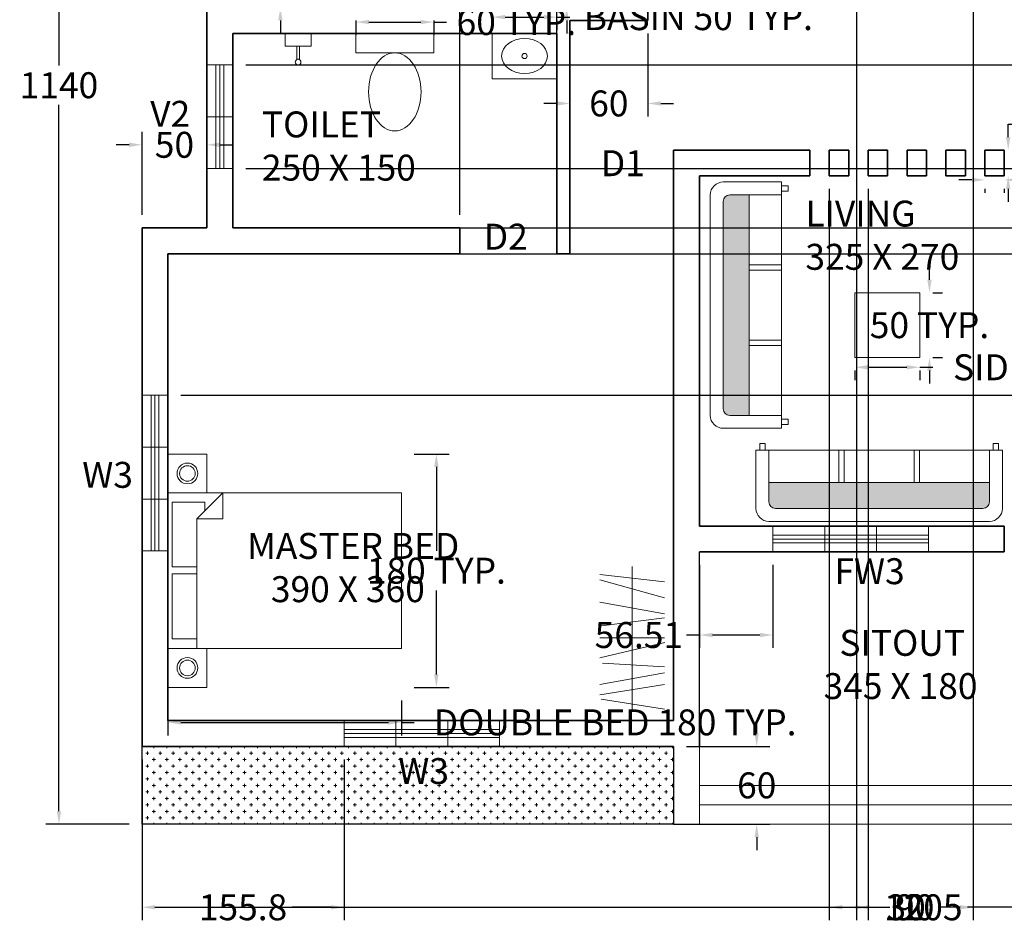
# Model space of a CAD drawing. Units: centimetres. Extents: x 543 to 2148, y 348 to 1642.
# Tile 1 of 4: x 543 to 1302, y 348 to 1046. Entities that reach past the tile are written whole.
import ezdxf

# ---------------------------------------------------------------- set-up
doc = ezdxf.new("R2010")
doc.units = ezdxf.units.CM
doc.header["$MEASUREMENT"] = 0
for name, color, linetype, lineweight in [('A-ANNO-DIMS', 2, 'Continuous', 18), ('A-ANNO-TEXT', 7, 'Continuous', 18), ('A-AREA-IDEN', 7, 'Continuous', 25), ('A-FLOR', 7, 'Continuous', 25), ('A-FLOR-CASE', 8, 'Continuous', 20), ('A-FLOR-FIXT', 8, 'Continuous', 18), ('A-FLOR-PATT', 252, 'Continuous', 13), ('A-FLOR-STRS', 7, 'Continuous', 20), ('A-FURN', 8, 'Continuous', 18), ('A-FURN-PATT', 252, 'Continuous', 13), ('A-GLAZ', 4, 'Continuous', 18), ('A-WALL', 7, 'Continuous', 35)]:
    doc.layers.add(name, color=color, linetype=linetype, lineweight=lineweight)
doc.styles.get("Standard").update_dxf_attribs({"font": 'arial.ttf'})
doc.dimstyles.get("Standard").update_dxf_attribs({"dimtxt": 20, "dimasz": 10, "dimexe": 10, "dimexo": 10, "dimgap": 5, "dimtad": 0, "dimtih": 1, "dimtoh": 1, "dimdec": 0, "dimzin": 0, "dimdsep": 46, "dimtxsty": 'Standard', "dimcen": 5, "dimadec": 0, "dimazin": 0, "dimtfac": 1, "dimtdec": 0, "dimtofl": 0, "dimtmove": 0, "dimatfit": 3, "dimfxl": 1, "dimtolj": 1, "dimtzin": 0, "dimarcsym": 0})

# ---------------------------------------------------------------- blocks, each defined once
blk = doc.blocks.new('BED-DOUBLE')
for p, q in [((42.36, 150), (22.36, 130)), ((42.36, 130), (42.36, 150)), ((22.36, 130), (22.36, 30)), ((22.36, 130), (42.36, 130)), ((3.32, 102.87), (3.32, 92.87)), ((3.32, 92.87), (22.36, 92.87)), ((3.32, 77.49), (3.32, 87.49)), ((3.32, 87.49), (22.36, 87.49))]:
    blk.add_line(p, q)
for points in [[(0, 150), (30, 150), (30, 180), (0, 180)], [(180, 150), (180, 30), (0, 30), (0, 150)], [(0, 0), (30, 0), (30, 30), (0, 30)]]:
    blk.add_lwpolyline(points, close=True)
for points in [[(3.32, 102.87), (3.32, 142.87), (28.32, 142.87), (28.32, 135.96)], [(22.36, 37.49), (3.32, 37.49), (3.32, 77.49)]]:
    blk.add_lwpolyline(points)
for centre, radius in [((15, 165), 8), ((15, 165), 6), ((15, 15), 8), ((15, 15), 6)]:
    blk.add_circle(centre, radius)
blk = doc.blocks.new('SOFA-3SEAT')
for p, q in [((10, 190), (55, 190)), ((55, 190), (55, 125.56)), ((55, 190), (55, 187)), ((55, 187), (60, 187)), ((60, 183), (55, 183)), ((60, 187), (60, 183)), ((0, 125.56), (0, 180)), ((10, 125.56), (10, 175)), ((15, 180), (55, 180)), ((30, 125.56), (30, 180)), ((0, 10), (0, 125.56)), ((10, 15), (10, 125.56)), ((55, 126), (30, 126)), ((30, 10), (30, 125.56)), ((55, 122), (30, 122)), ((55, 125.56), (55, 0)), ((55, 68), (30, 68)), ((55, 64), (30, 64)), ((55, 10), (15, 10)), ((55, 0), (10, 0)), ((60, 7), (55, 7)), ((55, 0), (55, 3)), ((55, 3), (60, 3)), ((60, 3), (60, 7))]:
    blk.add_line(p, q)
for centre, radius, start, end in [((10, 180), 10, 90, 180), ((15, 175), 5, 90, 180), ((10, 10), 10, 180, 270), ((15, 15), 5, 180, 270)]:
    blk.add_arc(centre, radius, start, end)
blk = doc.blocks.new('WARDROBE-RAIL')
for p, q in [((0, 0.31), (7.78, 49.18)), ((11.01, 50.31), (19.09, 0.31)), ((19.09, 50.31), (28.16, 0.3)), ((32.55, 0.31), (35.53, 48.25)), ((39.55, 50.31), (51.34, 0)), ((55, 0.31), (55, 50.31)), ((64.34, 49.01), (70.51, 0.27)), ((73.48, 0.31), (82.64, 50.31)), ((99.87, 50.31), (85.87, 0.31)), ((98.25, 0.31), (103.96, 50.31)), ((0, 25.31), (110, 25.31))]:
    blk.add_line(p, q)
blk = doc.blocks.new('WIN-1200')
for p, q in [((40, 20), (40, 0)), ((80, 20), (80, 0)), ((0, 13), (120, 13)), ((0, 10), (120, 10)), ((0, 7), (120, 7))]:
    blk.add_line(p, q)
blk.add_lwpolyline([(0, 20), (120, 20), (120, 0), (0, 0)], close=True)
blk = doc.blocks.new('VENT-800')
for p, q in [((7, 80), (7, 0)), ((10, 80), (10, 0)), ((13, 80), (13, 0)), ((20, 40), (0, 40)), ((20, 0), (0, 0))]:
    blk.add_line(p, q)
blk.add_lwpolyline([(0, 0), (0, 80), (20, 80), (20, 0)])
blk = doc.blocks.new('WC')
blk.add_lwpolyline([(60, 0), (0, 0), (0, 15), (60, 15)], close=True)
blk.add_ellipse((30, 45.11), major_axis=(0, 30.11), ratio=0.671585)
blk = doc.blocks.new('WASHBASIN')
blk.add_lwpolyline([(50, 0), (0, 0), (0, 35), (50, 35)], close=True)
blk.add_circle((25, 17.5), 2)
blk.add_ellipse((25, 17.5), major_axis=(17.65, 0), ratio=0.767259)
blk = doc.blocks.new('WALL-TAP')
for p, q in [((9, 10), (9, 20)), ((9, 20), (11, 20)), ((11, 10), (11, 20))]:
    blk.add_line(p, q)
blk.add_lwpolyline([(0, 0), (20, 0), (20, 10), (0, 10)], close=True)
blk.add_circle((10, 22.21), 2.21)
blk = doc.blocks.new('TABLE-SIDE')
blk.add_lwpolyline([(0, 50), (50, 50), (50, 0), (0, 0)], close=True)
blk = doc.blocks.new('SCREEN-POST-150X200')
for p, q in [((0, 0), (0, 20)), ((15, 20), (0, 20)), ((15, 0), (15, 20)), ((15, 0), (0, 0))]:
    blk.add_line(p, q)
blk = doc.blocks.new('*D17')
at = {"layer": 'A-ANNO-DIMS', "color": 0, "lineweight": -2, "transparency": 16777216}
for p, q in [((1305.14, 955.09), (1305.14, 965.09)), ((1305.14, 965.09), (1315.14, 965.09)), ((1312.14, 945.09), (1315.14, 945.09)), ((1312.14, 925.09), (1315.14, 925.09)), ((1305.14, 915.09), (1305.14, 905.09))]:
    blk.add_line(p, q, dxfattribs=at)
at = {"layer": 'A-ANNO-DIMS', "color": 0, "transparency": 16777216}
for points in [[(1303.47, 955.09), (1306.81, 955.09), (1305.14, 945.09)], [(1303.47, 915.09), (1306.81, 915.09), (1305.14, 925.09)]]:
    blk.add_solid(points, dxfattribs=at)
at = {"layer": 'Defpoints', "color": 0, "transparency": 16777216}
for p in [(1302.14, 945.09), (1305.14, 945.09), (1302.14, 925.09)]:
    blk.add_point(p, dxfattribs=at)
at = {"layer": 'A-ANNO-DIMS', "color": 0, "transparency": 16777216, "insert": (1472.79, 965.09), "char_height": 20, "attachment_point": 5}
blk.add_mtext('\\A1;SCREEN POST 20 TYP.', dxfattribs=at)
blk = doc.blocks.new('*D18')
at = {"layer": 'A-ANNO-DIMS', "color": 0, "lineweight": -2, "transparency": 16777216}
for p, q in [((1277.14, 922.09), (1267.14, 922.09)), ((1312.14, 922.09), (1322.14, 922.09)), ((1287.14, 915.09), (1287.14, 912.09)), ((1302.14, 915.09), (1302.14, 912.09))]:
    blk.add_line(p, q, dxfattribs=at)
at = {"layer": 'A-ANNO-DIMS', "color": 0, "transparency": 16777216}
for points in [[(1277.14, 923.76), (1277.14, 920.43), (1287.14, 922.09)], [(1312.14, 923.76), (1312.14, 920.43), (1302.14, 922.09)]]:
    blk.add_solid(points, dxfattribs=at)
at = {"layer": 'Defpoints', "color": 0, "transparency": 16777216}
for p in [(1287.14, 925.09), (1302.14, 925.09), (1302.14, 922.09)]:
    blk.add_point(p, dxfattribs=at)
at = {"layer": 'A-ANNO-DIMS', "color": 0, "transparency": 16777216, "insert": (1374.88, 922.09), "char_height": 20, "attachment_point": 5}
blk.add_mtext('\\A1;15 TYP.', dxfattribs=at)
blk = doc.blocks.new('*D21')
at = {"layer": 'A-ANNO-DIMS', "color": 0, "lineweight": -2, "transparency": 16777216}
for p, q in [((657.14, 520.66), (657.14, 493.66)), ((837.14, 520.66), (837.14, 493.66)), ((667.14, 503.66), (827.14, 503.66)), ((837.14, 503.66), (847.14, 503.66))]:
    blk.add_line(p, q, dxfattribs=at)
at = {"layer": 'A-ANNO-DIMS', "color": 0, "transparency": 16777216}
for points in [[(667.14, 505.32), (667.14, 501.99), (657.14, 503.66)], [(827.14, 505.32), (827.14, 501.99), (837.14, 503.66)]]:
    blk.add_solid(points, dxfattribs=at)
at = {"layer": 'Defpoints', "color": 0, "transparency": 16777216}
for p in [(657.14, 530.66), (837.14, 530.66), (837.14, 503.66)]:
    blk.add_point(p, dxfattribs=at)
at = {"layer": 'A-ANNO-DIMS', "color": 0, "transparency": 16777216, "insert": (1002.02, 503.66), "char_height": 20, "attachment_point": 5}
blk.add_mtext('\\A1;DOUBLE BED 180 TYP.', dxfattribs=at)
blk = doc.blocks.new('*D22')
at = {"layer": 'A-ANNO-DIMS', "color": 0, "lineweight": -2, "transparency": 16777216}
for p, q in [((847.14, 710.66), (874.14, 710.66)), ((864.14, 700.66), (864.14, 635.87)), ((864.14, 540.66), (864.14, 605.45)), ((847.14, 530.66), (874.14, 530.66))]:
    blk.add_line(p, q, dxfattribs=at)
at = {"layer": 'A-ANNO-DIMS', "color": 0, "transparency": 16777216}
for points in [[(862.47, 700.66), (865.81, 700.66), (864.14, 710.66)], [(862.47, 540.66), (865.81, 540.66), (864.14, 530.66)]]:
    blk.add_solid(points, dxfattribs=at)
at = {"layer": 'Defpoints', "color": 0, "transparency": 16777216}
for p in [(837.14, 710.66), (864.14, 710.66), (837.14, 530.66)]:
    blk.add_point(p, dxfattribs=at)
at = {"layer": 'A-ANNO-DIMS', "color": 0, "transparency": 16777216, "insert": (864.14, 620.66), "char_height": 20, "attachment_point": 5}
blk.add_mtext('\\A1;180 TYP.', dxfattribs=at)
blk = doc.blocks.new('*D30')
at = {"layer": 'A-ANNO-DIMS', "color": 0, "lineweight": -2, "transparency": 16777216}
for p, q in [((802.08, 1045.09), (802.08, 1033.81)), ((812.08, 1043.81), (852.08, 1043.81)), ((862.08, 1045.09), (862.08, 1033.81)), ((862.08, 1043.81), (872.08, 1043.81))]:
    blk.add_line(p, q, dxfattribs=at)
at = {"layer": 'A-ANNO-DIMS', "color": 0, "transparency": 16777216}
for points in [[(812.08, 1045.47), (812.08, 1042.14), (802.08, 1043.81)], [(852.08, 1045.47), (852.08, 1042.14), (862.08, 1043.81)]]:
    blk.add_solid(points, dxfattribs=at)
at = {"layer": 'Defpoints', "color": 0, "transparency": 16777216}
for p in [(802.08, 1055.09), (862.08, 1055.09), (862.08, 1043.81)]:
    blk.add_point(p, dxfattribs=at)
at = {"layer": 'A-ANNO-DIMS', "color": 0, "transparency": 16777216, "insert": (925.81, 1043.81), "char_height": 20, "attachment_point": 5}
blk.add_mtext('\\A1;60 TYP.', dxfattribs=at)
blk = doc.blocks.new('*D31')
at = {"layer": 'A-ANNO-DIMS', "color": 0, "lineweight": -2, "transparency": 16777216}
for p, q in [((907.14, 1045.09), (907.14, 1037.59)), ((917.14, 1047.59), (947.14, 1047.59)), ((957.14, 1047.59), (967.14, 1047.59)), ((957.14, 1045.09), (957.14, 1037.59))]:
    blk.add_line(p, q, dxfattribs=at)
at = {"layer": 'A-ANNO-DIMS', "color": 0, "transparency": 16777216}
for points in [[(917.14, 1049.26), (917.14, 1045.93), (907.14, 1047.59)], [(947.14, 1049.26), (947.14, 1045.93), (957.14, 1047.59)]]:
    blk.add_solid(points, dxfattribs=at)
at = {"layer": 'Defpoints', "color": 0, "transparency": 16777216}
for p in [(907.14, 1055.09), (957.14, 1055.09), (957.14, 1047.59)]:
    blk.add_point(p, dxfattribs=at)
at = {"layer": 'A-ANNO-DIMS', "color": 0, "transparency": 16777216, "insert": (1066.18, 1047.59), "char_height": 20, "attachment_point": 5}
blk.add_mtext('\\A1;BASIN 50 TYP.', dxfattribs=at)
blk = doc.blocks.new('*D32')
at = {"layer": 'A-ANNO-DIMS', "color": 0, "lineweight": -2, "transparency": 16777216}
for p, q in [((964.64, 1100.09), (964.64, 1110.09)), ((967.14, 1090.09), (974.64, 1090.09)), ((967.14, 1055.09), (974.64, 1055.09)), ((964.64, 1045.09), (964.64, 1035.09))]:
    blk.add_line(p, q, dxfattribs=at)
at = {"layer": 'A-ANNO-DIMS', "color": 0, "transparency": 16777216}
for points in [[(962.97, 1100.09), (966.31, 1100.09), (964.64, 1090.09)], [(962.97, 1045.09), (966.31, 1045.09), (964.64, 1055.09)]]:
    blk.add_solid(points, dxfattribs=at)
at = {"layer": 'Defpoints', "color": 0, "transparency": 16777216}
for p in [(957.14, 1090.09), (964.64, 1090.09), (957.14, 1055.09)]:
    blk.add_point(p, dxfattribs=at)
at = {"layer": 'A-ANNO-DIMS', "color": 0, "transparency": 16777216, "insert": (964.64, 1072.59), "char_height": 20, "attachment_point": 5}
blk.add_mtext('\\A1;35 TYP.', dxfattribs=at)
blk = doc.blocks.new('*D33')
at = {"layer": 'A-ANNO-DIMS', "color": 0, "lineweight": -2, "transparency": 16777216}
for p, q in [((743.83, 1089.51), (743.83, 1099.51)), ((743.83, 1099.51), (753.83, 1099.51)), ((737.5, 1079.51), (733.83, 1079.51)), ((737.5, 1055.09), (733.83, 1055.09)), ((743.83, 1045.09), (743.83, 1035.09))]:
    blk.add_line(p, q, dxfattribs=at)
at = {"layer": 'A-ANNO-DIMS', "color": 0, "transparency": 16777216}
for points in [[(742.17, 1089.51), (745.5, 1089.51), (743.83, 1079.51)], [(742.17, 1045.09), (745.5, 1045.09), (743.83, 1055.09)]]:
    blk.add_solid(points, dxfattribs=at)
at = {"layer": 'Defpoints', "color": 0, "transparency": 16777216}
for p in [(743.83, 1079.51), (747.5, 1079.51), (747.5, 1055.09)]:
    blk.add_point(p, dxfattribs=at)
at = {"layer": 'A-ANNO-DIMS', "color": 0, "transparency": 16777216, "insert": (838.81, 1099.51), "char_height": 20, "attachment_point": 5}
blk.add_mtext('\\A1;TAP 24 TYP.', dxfattribs=at)
blk = doc.blocks.new('*D35')
at = {"layer": 'A-ANNO-DIMS', "color": 0, "lineweight": -2, "transparency": 16777216}
for p, q in [((1186.93, 775.04), (1186.93, 767.54)), ((1196.93, 777.54), (1226.93, 777.54)), ((1236.93, 777.54), (1246.93, 777.54)), ((1236.93, 775.04), (1236.93, 767.54))]:
    blk.add_line(p, q, dxfattribs=at)
at = {"layer": 'A-ANNO-DIMS', "color": 0, "transparency": 16777216}
for points in [[(1196.93, 779.21), (1196.93, 775.87), (1186.93, 777.54)], [(1226.93, 779.21), (1226.93, 775.87), (1236.93, 777.54)]]:
    blk.add_solid(points, dxfattribs=at)
at = {"layer": 'Defpoints', "color": 0, "transparency": 16777216}
for p in [(1186.93, 785.04), (1236.93, 785.04), (1236.93, 777.54)]:
    blk.add_point(p, dxfattribs=at)
at = {"layer": 'A-ANNO-DIMS', "color": 0, "transparency": 16777216, "insert": (1385.19, 777.54), "char_height": 20, "attachment_point": 5}
blk.add_mtext('\\A1;SIDE TABLE 50 TYP.', dxfattribs=at)
blk = doc.blocks.new('*D36')
at = {"layer": 'A-ANNO-DIMS', "color": 0, "lineweight": -2, "transparency": 16777216}
for p, q in [((1244.43, 845.04), (1244.43, 855.04)), ((1246.93, 835.04), (1254.43, 835.04)), ((1246.93, 785.04), (1254.43, 785.04)), ((1244.43, 775.04), (1244.43, 765.04))]:
    blk.add_line(p, q, dxfattribs=at)
at = {"layer": 'A-ANNO-DIMS', "color": 0, "transparency": 16777216}
for points in [[(1242.77, 845.04), (1246.1, 845.04), (1244.43, 835.04)], [(1242.77, 775.04), (1246.1, 775.04), (1244.43, 785.04)]]:
    blk.add_solid(points, dxfattribs=at)
at = {"layer": 'Defpoints', "color": 0, "transparency": 16777216}
for p in [(1236.93, 835.04), (1244.43, 835.04), (1236.93, 785.04)]:
    blk.add_point(p, dxfattribs=at)
at = {"layer": 'A-ANNO-DIMS', "color": 0, "transparency": 16777216, "insert": (1244.43, 810.04), "char_height": 20, "attachment_point": 5}
blk.add_mtext('\\A1;50 TYP.', dxfattribs=at)
blk = doc.blocks.new('*D37')
at = {"layer": 'A-ANNO-DIMS', "color": 0, "lineweight": -2, "transparency": 16777216}
for p, q in [((637.14, 895.09), (637.14, 959.14)), ((687.14, 895.09), (687.14, 959.14)), ((627.14, 949.14), (617.14, 949.14)), ((697.14, 949.14), (707.14, 949.14))]:
    blk.add_line(p, q, dxfattribs=at)
at = {"layer": 'A-ANNO-DIMS', "color": 0, "transparency": 16777216}
for points in [[(627.14, 950.81), (627.14, 947.48), (637.14, 949.14)], [(697.14, 950.81), (697.14, 947.48), (687.14, 949.14)]]:
    blk.add_solid(points, dxfattribs=at)
at = {"layer": 'Defpoints', "color": 0, "transparency": 16777216}
for p in [(687.14, 949.14), (637.14, 885.09), (687.14, 885.09)]:
    blk.add_point(p, dxfattribs=at)
at = {"layer": 'A-ANNO-DIMS', "color": 0, "transparency": 16777216, "insert": (662.14, 949.14), "char_height": 20, "attachment_point": 5}
blk.add_mtext('\\A1;50', dxfattribs=at)
blk = doc.blocks.new('*D44')
at = {"layer": 'A-ANNO-DIMS', "color": 0, "lineweight": -2, "transparency": 16777216}
for p, q in [((882.14, 895.09), (882.14, 1639.14)), ((957.14, 895.09), (957.14, 1639.14)), ((892.14, 1629.14), (900.32, 1629.14)), ((947.14, 1629.14), (938.96, 1629.14))]:
    blk.add_line(p, q, dxfattribs=at)
at = {"layer": 'A-ANNO-DIMS', "color": 0, "transparency": 16777216}
for points in [[(892.14, 1630.81), (892.14, 1627.48), (882.14, 1629.14)], [(947.14, 1630.81), (947.14, 1627.48), (957.14, 1629.14)]]:
    blk.add_solid(points, dxfattribs=at)
at = {"layer": 'Defpoints', "color": 0, "transparency": 16777216}
for p in [(957.14, 1629.14), (882.14, 885.09), (957.14, 885.09)]:
    blk.add_point(p, dxfattribs=at)
at = {"layer": 'A-ANNO-DIMS', "color": 0, "transparency": 16777216, "insert": (919.64, 1629.14), "char_height": 20, "attachment_point": 5}
blk.add_mtext('\\A1;75', dxfattribs=at)
blk = doc.blocks.new('*D46')
at = {"layer": 'A-ANNO-DIMS', "color": 0, "lineweight": -2, "transparency": 16777216}
for p, q in [((1111.19, 495.09), (1111.19, 505.09)), ((1057.14, 485.09), (1121.19, 485.09)), ((1057.14, 425.09), (1121.19, 425.09)), ((1111.19, 415.09), (1111.19, 405.09))]:
    blk.add_line(p, q, dxfattribs=at)
at = {"layer": 'A-ANNO-DIMS', "color": 0, "transparency": 16777216}
for points in [[(1109.52, 495.09), (1112.86, 495.09), (1111.19, 485.09)], [(1109.52, 415.09), (1112.86, 415.09), (1111.19, 425.09)]]:
    blk.add_solid(points, dxfattribs=at)
at = {"layer": 'Defpoints', "color": 0, "transparency": 16777216}
for p in [(1047.14, 485.09), (1047.14, 425.09), (1111.19, 425.09)]:
    blk.add_point(p, dxfattribs=at)
at = {"layer": 'A-ANNO-DIMS', "color": 0, "transparency": 16777216, "insert": (1111.19, 455.09), "char_height": 20, "attachment_point": 5}
blk.add_mtext('\\A1;60', dxfattribs=at)
blk = doc.blocks.new('*D55')
at = {"layer": 'A-ANNO-DIMS', "color": 0, "lineweight": -2, "transparency": 16777216}
for p, q in [((1067.14, 625.09), (1067.14, 561.04)), ((1123.65, 625.09), (1123.65, 561.04)), ((1067.14, 571.04), (1057.14, 571.04)), ((1113.65, 571.04), (1077.14, 571.04))]:
    blk.add_line(p, q, dxfattribs=at)
at = {"layer": 'A-ANNO-DIMS', "color": 0, "transparency": 16777216}
for points in [[(1077.14, 572.71), (1077.14, 569.38), (1067.14, 571.04)], [(1113.65, 572.71), (1113.65, 569.38), (1123.65, 571.04)]]:
    blk.add_solid(points, dxfattribs=at)
at = {"layer": 'Defpoints', "color": 0, "transparency": 16777216}
for p in [(1067.14, 635.09), (1123.65, 635.09), (1067.14, 571.04)]:
    blk.add_point(p, dxfattribs=at)
at = {"layer": 'A-ANNO-DIMS', "color": 0, "transparency": 16777216, "insert": (1020.33, 571.04), "char_height": 20, "attachment_point": 5}
blk.add_mtext('\\A1;56.51', dxfattribs=at)
blk = doc.blocks.new('*D56')
at = {"layer": 'A-ANNO-DIMS', "color": 0, "lineweight": -2, "transparency": 16777216}
for p, q in [((637.14, 475.09), (637.14, 351.04)), ((792.95, 475.09), (792.95, 351.04)), ((647.14, 361.04), (677.22, 361.04)), ((782.95, 361.04), (752.87, 361.04))]:
    blk.add_line(p, q, dxfattribs=at)
at = {"layer": 'A-ANNO-DIMS', "color": 0, "transparency": 16777216}
for points in [[(647.14, 362.71), (647.14, 359.38), (637.14, 361.04)], [(782.95, 362.71), (782.95, 359.38), (792.95, 361.04)]]:
    blk.add_solid(points, dxfattribs=at)
at = {"layer": 'Defpoints', "color": 0, "transparency": 16777216}
for p in [(637.14, 485.09), (792.95, 485.09), (792.95, 361.04)]:
    blk.add_point(p, dxfattribs=at)
at = {"layer": 'A-ANNO-DIMS', "color": 0, "transparency": 16777216, "insert": (715.05, 361.04), "char_height": 20, "attachment_point": 5}
blk.add_mtext('\\A1;155.8', dxfattribs=at)
blk = doc.blocks.new('*D57')
at = {"layer": 'A-ANNO-DIMS', "color": 0, "lineweight": -2, "transparency": 16777216}
for p, q in [((667.14, 865.09), (1916.19, 865.09)), ((1906.19, 855.09), (1906.19, 825.73)), ((1906.19, 765.94), (1906.19, 795.31)), ((667.14, 755.94), (1916.19, 755.94))]:
    blk.add_line(p, q, dxfattribs=at)
at = {"layer": 'A-ANNO-DIMS', "color": 0, "transparency": 16777216}
for points in [[(1904.52, 855.09), (1907.86, 855.09), (1906.19, 865.09)], [(1904.52, 765.94), (1907.86, 765.94), (1906.19, 755.94)]]:
    blk.add_solid(points, dxfattribs=at)
at = {"layer": 'Defpoints', "color": 0, "transparency": 16777216}
for p in [(657.14, 865.09), (657.14, 755.94), (1906.19, 755.94)]:
    blk.add_point(p, dxfattribs=at)
at = {"layer": 'A-ANNO-DIMS', "color": 0, "transparency": 16777216, "insert": (1906.19, 810.52), "char_height": 20, "attachment_point": 5}
blk.add_mtext('\\A1;109.15', dxfattribs=at)
blk = doc.blocks.new('*D58')
at = {"layer": 'A-ANNO-DIMS', "color": 0, "lineweight": -2, "transparency": 16777216}
for p, q in [((1906.19, 940.76), (1906.19, 950.76)), ((717.14, 930.76), (1916.19, 930.76)), ((717.14, 885.09), (1916.19, 885.09)), ((1906.19, 875.09), (1906.19, 865.09))]:
    blk.add_line(p, q, dxfattribs=at)
at = {"layer": 'A-ANNO-DIMS', "color": 0, "transparency": 16777216}
for points in [[(1904.52, 940.76), (1907.86, 940.76), (1906.19, 930.76)], [(1904.52, 875.09), (1907.86, 875.09), (1906.19, 885.09)]]:
    blk.add_solid(points, dxfattribs=at)
at = {"layer": 'Defpoints', "color": 0, "transparency": 16777216}
for p in [(707.14, 930.76), (1906.19, 930.76), (707.14, 885.09)]:
    blk.add_point(p, dxfattribs=at)
at = {"layer": 'A-ANNO-DIMS', "color": 0, "transparency": 16777216, "insert": (1906.19, 907.92), "char_height": 20, "attachment_point": 5}
blk.add_mtext('\\A1;45.67', dxfattribs=at)
blk = doc.blocks.new('*D59')
at = {"layer": 'A-ANNO-DIMS', "color": 0, "lineweight": -2, "transparency": 16777216}
for p, q in [((717.14, 1089.08), (1916.19, 1089.08)), ((1906.19, 1079.08), (1906.19, 1065.14)), ((1906.19, 1020.76), (1906.19, 1034.7)), ((717.14, 1010.76), (1916.19, 1010.76))]:
    blk.add_line(p, q, dxfattribs=at)
at = {"layer": 'A-ANNO-DIMS', "color": 0, "transparency": 16777216}
for points in [[(1904.52, 1079.08), (1907.86, 1079.08), (1906.19, 1089.08)], [(1904.52, 1020.76), (1907.86, 1020.76), (1906.19, 1010.76)]]:
    blk.add_solid(points, dxfattribs=at)
at = {"layer": 'Defpoints', "color": 0, "transparency": 16777216}
for p in [(707.14, 1089.08), (1906.19, 1089.08), (707.14, 1010.76)]:
    blk.add_point(p, dxfattribs=at)
at = {"layer": 'A-ANNO-DIMS', "color": 0, "transparency": 16777216, "insert": (1906.19, 1049.92), "char_height": 20, "attachment_point": 5}
blk.add_mtext('\\A1;78.33', dxfattribs=at)
blk = doc.blocks.new('*D64')
at = {"layer": 'A-ANNO-DIMS', "color": 0, "lineweight": -2, "transparency": 16777216}
for p, q in [((1188.09, 1079.31), (1188.09, 351.04)), ((1278.09, 1079.31), (1278.09, 351.04)), ((1198.09, 361.04), (1213.8, 361.04)), ((1268.09, 361.04), (1252.38, 361.04))]:
    blk.add_line(p, q, dxfattribs=at)
at = {"layer": 'A-ANNO-DIMS', "color": 0, "transparency": 16777216}
for points in [[(1198.09, 362.71), (1198.09, 359.38), (1188.09, 361.04)], [(1268.09, 362.71), (1268.09, 359.38), (1278.09, 361.04)]]:
    blk.add_solid(points, dxfattribs=at)
at = {"layer": 'Defpoints', "color": 0, "transparency": 16777216}
for p in [(1188.09, 1089.31), (1278.09, 1089.31), (1278.09, 361.04)]:
    blk.add_point(p, dxfattribs=at)
at = {"layer": 'A-ANNO-DIMS', "color": 0, "transparency": 16777216, "insert": (1233.09, 361.04), "char_height": 20, "attachment_point": 5}
blk.add_mtext('\\A1;90', dxfattribs=at)
blk = doc.blocks.new('*D66')
at = {"layer": 'A-ANNO-DIMS', "color": 0, "lineweight": -2, "transparency": 16777216}
for p, q in [((1167.14, 915.09), (1167.14, 351.04)), ((1197.14, 915.09), (1197.14, 351.04)), ((1177.14, 361.04), (1187.14, 361.04)), ((1197.14, 361.04), (1207.14, 361.04))]:
    blk.add_line(p, q, dxfattribs=at)
at = {"layer": 'A-ANNO-DIMS', "color": 0, "transparency": 16777216}
for points in [[(1177.14, 362.71), (1177.14, 359.38), (1167.14, 361.04)], [(1187.14, 362.71), (1187.14, 359.38), (1197.14, 361.04)]]:
    blk.add_solid(points, dxfattribs=at)
at = {"layer": 'Defpoints', "color": 0, "transparency": 16777216}
for p in [(1167.14, 925.09), (1197.14, 925.09), (1197.14, 361.04)]:
    blk.add_point(p, dxfattribs=at)
at = {"layer": 'A-ANNO-DIMS', "color": 0, "transparency": 16777216, "insert": (1226.42, 361.04), "char_height": 20, "attachment_point": 5}
blk.add_mtext('\\A1;30', dxfattribs=at)
blk = doc.blocks.new('*D67')
at = {"layer": 'A-ANNO-DIMS', "color": 0, "lineweight": -2, "transparency": 16777216}
for p, q in [((677.14, 1565.09), (563.09, 1565.09)), ((573.09, 1555.09), (573.09, 1010.3)), ((573.09, 435.09), (573.09, 979.88)), ((627.14, 425.09), (563.09, 425.09))]:
    blk.add_line(p, q, dxfattribs=at)
at = {"layer": 'A-ANNO-DIMS', "color": 0, "transparency": 16777216}
for points in [[(571.42, 1555.09), (574.76, 1555.09), (573.09, 1565.09)], [(571.42, 435.09), (574.76, 435.09), (573.09, 425.09)]]:
    blk.add_solid(points, dxfattribs=at)
at = {"layer": 'Defpoints', "color": 0, "transparency": 16777216}
for p in [(573.09, 1565.09), (687.14, 1565.09), (637.14, 425.09)]:
    blk.add_point(p, dxfattribs=at)
at = {"layer": 'A-ANNO-DIMS', "color": 0, "transparency": 16777216, "insert": (573.09, 995.09), "char_height": 20, "attachment_point": 5}
blk.add_mtext('\\A1;1140', dxfattribs=at)
blk = doc.blocks.new('*D68')
at = {"layer": 'A-ANNO-DIMS', "color": 0, "lineweight": -2, "transparency": 16777216}
for p, q in [((1842.14, 1185.09), (1842.14, 351.04)), ((637.14, 415.09), (637.14, 351.04)), ((647.14, 361.04), (1205.64, 361.04)), ((1832.14, 361.04), (1273.64, 361.04))]:
    blk.add_line(p, q, dxfattribs=at)
at = {"layer": 'A-ANNO-DIMS', "color": 0, "transparency": 16777216}
for points in [[(647.14, 362.71), (647.14, 359.38), (637.14, 361.04)], [(1832.14, 362.71), (1832.14, 359.38), (1842.14, 361.04)]]:
    blk.add_solid(points, dxfattribs=at)
at = {"layer": 'Defpoints', "color": 0, "transparency": 16777216}
for p in [(1842.14, 1195.09), (637.14, 425.09), (1842.14, 361.04)]:
    blk.add_point(p, dxfattribs=at)
at = {"layer": 'A-ANNO-DIMS', "color": 0, "transparency": 16777216, "insert": (1239.64, 361.04), "char_height": 20, "attachment_point": 5}
blk.add_mtext('\\A1;1205', dxfattribs=at)
blk = doc.blocks.new('*D73')
at = {"layer": 'A-ANNO-DIMS', "color": 0, "lineweight": -2, "transparency": 16777216}
for p, q in [((967.14, 1035.09), (967.14, 971.04)), ((1027.14, 1035.09), (1027.14, 971.04)), ((957.14, 981.04), (947.14, 981.04)), ((1037.14, 981.04), (1047.14, 981.04))]:
    blk.add_line(p, q, dxfattribs=at)
at = {"layer": 'A-ANNO-DIMS', "color": 0, "transparency": 16777216}
for points in [[(957.14, 982.71), (957.14, 979.38), (967.14, 981.04)], [(1037.14, 982.71), (1037.14, 979.38), (1027.14, 981.04)]]:
    blk.add_solid(points, dxfattribs=at)
at = {"layer": 'Defpoints', "color": 0, "transparency": 16777216}
for p in [(967.14, 1045.09), (1027.14, 1045.09), (967.14, 981.04)]:
    blk.add_point(p, dxfattribs=at)
at = {"layer": 'A-ANNO-DIMS', "color": 0, "transparency": 16777216, "insert": (997.14, 981.04), "char_height": 20, "attachment_point": 5}
blk.add_mtext('\\A1;60', dxfattribs=at)

msp = doc.modelspace()

# ---------------------------------------------------------------- hatches: boundary and pattern name
at = {"layer": 'A-FLOR-PATT'}
h = msp.add_hatch(dxfattribs=at)
h.set_pattern_fill('CROSS', color=256, scale=20)
h.paths.add_polyline_path([(1047.141, 485.092), (637.141, 485.092), (637.141, 425.092), (1047.141, 425.092), (1047.141, 455.092)])
h.paths.add_polyline_path([(829.385, 445.104), (881.295, 445.104), (881.295, 486.319), (829.385, 486.319)], flags=9)
at = {"layer": 'A-FURN-PATT'}
h = msp.add_hatch(dxfattribs=at)
h.set_pattern_fill('CROSS', color=256, scale=25)
h.paths.add_polyline_path([(1290.635, 688.693), (1175.07, 688.693), (1120.635, 688.693), (1120.635, 673.693, 0.4142136), (1125.635, 668.693), (1175.07, 668.693), (1285.635, 668.693, 0.4142136), (1290.635, 673.693)])
h.paths.add_polyline_path([(1105.412, 856.024), (1105.412, 910.459), (1090.412, 910.459, 0.4142136), (1085.412, 905.459), (1085.412, 856.024), (1085.412, 745.459, 0.4142136), (1090.412, 740.459), (1105.412, 740.459)])
h.paths.add_polyline_path([(1126.48, 1465.069), (1126.48, 1519.504), (1111.48, 1519.504, 0.4142136), (1106.48, 1514.504), (1106.48, 1465.069), (1106.48, 1354.504, 0.4142136), (1111.48, 1349.504), (1126.48, 1349.504)])

# ---------------------------------------------------------------- linework, layer by layer
at = {"layer": 'A-FLOR'}
for p, q in [((1067.141, 485.092), (1067.141, 635.092)), ((637.141, 425.092), (637.141, 485.092)), ((1047.141, 485.092), (1047.141, 455.092)), ((1047.141, 455.092), (1047.141, 425.092)), ((1047.141, 425.092), (637.141, 425.092)), ((1047.141, 425.092), (1067.141, 425.092))]:
    msp.add_line(p, q, dxfattribs=at)
at = {"layer": 'A-FLOR-STRS'}
for p, q in [((1067.141, 485.092), (1067.141, 425.092)), ((1067.141, 455.092), (1432.141, 455.092)), ((1067.141, 440.092), (1432.141, 440.092)), ((1067.141, 425.092), (1432.141, 425.092))]:
    msp.add_line(p, q, dxfattribs=at)
at = {"layer": 'A-WALL'}
for p, q in [((687.141, 1565.092), (687.141, 885.092)), ((1027.141, 1055.092), (1027.141, 1045.092)), ((967.141, 865.092), (967.141, 1045.092)), ((1027.141, 1045.092), (967.141, 1045.092)), ((707.141, 1035.092), (957.141, 1035.092)), ((707.141, 885.092), (707.141, 1035.092)), ((957.141, 1035.092), (957.141, 885.092)), ((1047.141, 865.092), (1047.141, 945.092)), ((1047.141, 945.092), (1067.141, 945.092)), ((1152.141, 945.092), (1067.141, 945.092)), ((1152.141, 925.092), (1152.141, 945.092)), ((1242.141, 925.092), (1242.141, 945.092)), ((1067.141, 655.092), (1067.141, 925.092)), ((1152.141, 925.092), (1067.141, 925.092)), ((687.141, 885.092), (637.141, 885.092)), ((637.141, 885.092), (637.141, 865.092)), ((882.141, 885.092), (707.141, 885.092)), ((882.141, 885.092), (882.141, 865.092)), ((957.141, 885.092), (957.141, 865.092)), ((637.141, 865.092), (637.141, 485.092)), ((657.141, 865.092), (687.141, 865.092)), ((657.141, 865.092), (882.141, 865.092)), ((657.141, 505.092), (657.141, 865.092)), ((687.141, 865.092), (707.141, 865.092)), ((957.141, 865.092), (967.141, 865.092)), ((1047.141, 865.092), (1047.141, 505.092)), ((1302.141, 655.092), (1067.141, 655.092)), ((1302.141, 655.092), (1302.141, 635.092)), ((1302.141, 635.092), (1067.141, 635.092)), ((1047.141, 505.092), (657.141, 505.092)), ((1067.141, 505.092), (1067.141, 485.092)), ((637.141, 485.092), (1047.141, 485.092))]:
    msp.add_line(p, q, dxfattribs=at)

# ---------------------------------------------------------------- block references
at = {"layer": 'A-FLOR-CASE', "rotation": 90.00000000000011}
msp.add_blockref('WARDROBE-RAIL', (1040.461, 513.827), dxfattribs=at)
at = {"layer": 'A-FLOR-FIXT', "extrusion": (0, 0, -1), "zscale": -1, "rotation": 180}
for name, p in [('WALL-TAP', (-747.497, 1035.092)), ('WC', (-802.082, 1035.092)), ('WASHBASIN', (-907.141, 1035.092))]:
    msp.add_blockref(name, p, dxfattribs=at)
at = {"layer": 'A-FURN'}
for name, p in [('SOFA-3SEAT', (1075.412, 730.459)), ('TABLE-SIDE', (1186.933, 785.039)), ('BED-DOUBLE', (657.141, 530.658))]:
    msp.add_blockref(name, p, dxfattribs=at)
at = {"layer": 'A-FURN', "rotation": 89.99999999999966}
msp.add_blockref('SOFA-3SEAT', (1300.635, 658.693), dxfattribs=at)
at = {"layer": 'A-GLAZ'}
for name, p in [('VENT-800', (687.141, 930.758)), ('WIN-1200', (1123.649, 635.092)), ('WIN-1200', (792.951, 485.092))]:
    msp.add_blockref(name, p, dxfattribs=at)
at = {"layer": 'A-GLAZ', "rotation": 270.0000000000002}
msp.add_blockref('WIN-1200', (637.141, 755.945), dxfattribs=at)
at = {"layer": 'A-WALL'}
for p in [(1167.141, 925.092), (1197.141, 925.092), (1227.141, 925.092), (1257.141, 925.092), (1287.141, 925.092)]:
    msp.add_blockref('SCREEN-POST-150X200', p, dxfattribs=at)

# ---------------------------------------------------------------- texts
at = {"layer": 'A-ANNO-TEXT', "char_height": 20, "attachment_point": 1}
for s, insert in [('V2', (643.484, 983.026)), ('D1', (991.038, 944.934)), ('D2', (900.72, 888.267)), ('W3', (591.038, 704.584)), ('FW3', (1171.136, 630.268)), ('W3', (834.727, 476.107))]:
    msp.add_mtext_dynamic_manual_height_columns(s, width=246.06417, gutter_width=1, heights=[0], dxfattribs=dict(at, insert=insert))
at = {"layer": 'A-AREA-IDEN', "char_height": 20, "attachment_point": 1}
for s, insert in [('TOILET\\P250 X 150', (729.6, 974.858)), ('LIVING\\P325 X 270', (1148.71, 906.075)), ('MASTER BED\\P   390 X 360', (718.19, 649.734)), ('  SITOUT\\P345 X 180', (1162.758, 574.996))]:
    msp.add_mtext_dynamic_manual_height_columns(s, width=246.06417, gutter_width=1, heights=[0], dxfattribs=dict(at, insert=insert))

# ---------------------------------------------------------------- dimensions: what is measured, and where the dimension line sits
at = {"layer": 'A-ANNO-DIMS'}
for base, p1, p2, override, picture, middle in [((957.141, 1629.142), (882.141, 885.092), (957.141, 885.092), {"dimdec": 0, "dimlfac": 1, "dimrnd": 0, "dimzin": 0, "dimdsep": 46, "dimlunit": 2}, '*D44', (919.641, 1629.142)), ((1842.141, 361.042), (637.141, 425.092), (1842.141, 1195.092), {"dimdec": 0, "dimlfac": 1, "dimrnd": 0, "dimzin": 0, "dimdsep": 46, "dimlunit": 2}, '*D68', (1239.641, 361.042)), ((1278.094, 361.042), (1188.094, 1089.313), (1278.094, 1089.313), {"dimdec": 0, "dimlfac": 1, "dimrnd": 0, "dimzin": 0, "dimdsep": 46, "dimlunit": 2}, '*D64', (1233.094, 361.042)), ((687.141, 949.142), (637.141, 885.092), (687.141, 885.092), {"dimdec": 0, "dimlfac": 1, "dimrnd": 0, "dimzin": 0, "dimdsep": 46, "dimlunit": 2}, '*D37', (662.141, 949.142)), ((1197.141, 361.042), (1167.141, 925.092), (1197.141, 925.092), {"dimdec": 0, "dimlfac": 1, "dimrnd": 0, "dimzin": 0, "dimdsep": 46, "dimlunit": 2}, '*D66', (1226.425, 361.042)), ((792.951, 361.042), (637.141, 485.092), (792.951, 485.092), {"dimdec": 1, "dimlfac": 1, "dimrnd": 0, "dimzin": 0, "dimdsep": 46, "dimlunit": 2}, '*D56', (715.046, 361.042))]:
    dim = msp.add_linear_dim(base=base, p1=p1, p2=p2, dimstyle='Standard', override=override, dxfattribs=at)
    dim.commit()
    dim.dimension.update_dxf_attribs({"geometry": picture, "text_midpoint": middle})
for base, p1, p2, angle, override, picture, middle in [((573.091, 1565.092), (637.141, 425.092), (687.141, 1565.092), 90, {"dimdec": 0, "dimlfac": 1, "dimrnd": 0, "dimzin": 0, "dimdsep": 46, "dimlunit": 2}, '*D67', (573.091, 995.092)), ((1906.1909, 1089.0833), (707.1409, 1010.7581), (707.1409, 1089.0833), 90, {"dimdec": 2, "dimlfac": 1, "dimrnd": 0, "dimzin": 0, "dimdsep": 46, "dimlunit": 2}, '*D59', (1906.1909, 1049.9207)), ((967.141, 981.042), (1027.141, 1045.092), (967.141, 1045.092), 180, {"dimdec": 0, "dimlfac": 1, "dimrnd": 0, "dimzin": 0, "dimdsep": 46, "dimlunit": 2}, '*D73', (997.141, 981.042)), ((1906.191, 930.758), (707.141, 885.092), (707.141, 930.758), 90, {"dimdec": 2, "dimlfac": 1, "dimrnd": 0, "dimzin": 0, "dimdsep": 46, "dimlunit": 2}, '*D58', (1906.191, 907.925)), ((1906.191, 755.945), (657.141, 865.092), (657.141, 755.945), 90, {"dimdec": 2, "dimlfac": 1, "dimrnd": 0, "dimzin": 0, "dimdsep": 46, "dimlunit": 2}, '*D57', (1906.191, 810.518)), ((1067.141, 571.042), (1123.649, 635.092), (1067.141, 635.092), 180, {"dimdec": 2, "dimlfac": 1, "dimrnd": 0, "dimzin": 0, "dimdsep": 46, "dimlunit": 2}, '*D55', (1020.326, 571.042)), ((1111.191, 425.092), (1047.141, 485.092), (1047.141, 425.092), 270, {"dimdec": 0, "dimlfac": 1, "dimrnd": 0, "dimzin": 0, "dimdsep": 46, "dimlunit": 2}, '*D46', (1111.191, 455.092))]:
    dim = msp.add_linear_dim(base=base, p1=p1, p2=p2, angle=angle, dimstyle='Standard', override=override, dxfattribs=at)
    dim.commit()
    dim.dimension.update_dxf_attribs({"geometry": picture, "text_midpoint": middle})
for base, p1, p2, text, picture, middle in [((743.834, 1079.513), (747.497, 1055.092), (747.497, 1079.513), 'TAP <> TYP.', '*D33', (838.814, 1099.513)), ((964.641, 1090.092), (957.141, 1055.092), (957.141, 1090.092), '<> TYP.', '*D32', (964.641, 1072.592)), ((1305.141, 945.092), (1302.141, 925.092), (1302.141, 945.092), 'SCREEN POST <> TYP.', '*D17', (1472.788, 965.092)), ((1244.433, 835.039), (1236.933, 785.039), (1236.933, 835.039), '<> TYP.', '*D36', (1244.433, 810.039)), ((864.141, 710.658), (837.141, 530.658), (837.141, 710.658), '<> TYP.', '*D22', (864.141, 620.658))]:
    dim = msp.add_linear_dim(base=base, p1=p1, p2=p2, angle=90, text=text, dimstyle='Standard', override={"dimdec": 0, "dimlfac": 1, "dimrnd": 0, "dimzin": 0, "dimdsep": 46, "dimlunit": 2}, dxfattribs=at)
    dim.commit()
    dim.dimension.update_dxf_attribs({"geometry": picture, "text_midpoint": middle})
for base, p1, p2, text, picture, middle in [((957.141, 1047.592), (907.141, 1055.092), (957.141, 1055.092), 'BASIN <> TYP.', '*D31', (1066.179, 1047.592)), ((862.082, 1043.808), (802.082, 1055.092), (862.082, 1055.092), '<> TYP.', '*D30', (925.813, 1043.808)), ((1302.141, 922.092), (1287.141, 925.092), (1302.141, 925.092), '<> TYP.', '*D18', (1374.876, 922.092)), ((1236.933, 777.539), (1186.933, 785.039), (1236.933, 785.039), 'SIDE TABLE <> TYP.', '*D35', (1385.187, 777.539)), ((837.141, 503.658), (657.141, 530.658), (837.141, 530.658), 'DOUBLE BED <> TYP.', '*D21', (1002.025, 503.658))]:
    dim = msp.add_linear_dim(base=base, p1=p1, p2=p2, text=text, dimstyle='Standard', override={"dimdec": 0, "dimlfac": 1, "dimrnd": 0, "dimzin": 0, "dimdsep": 46, "dimlunit": 2}, dxfattribs=at)
    dim.commit()
    dim.dimension.update_dxf_attribs({"geometry": picture, "text_midpoint": middle})

doc.saveas('drawing.dxf')
